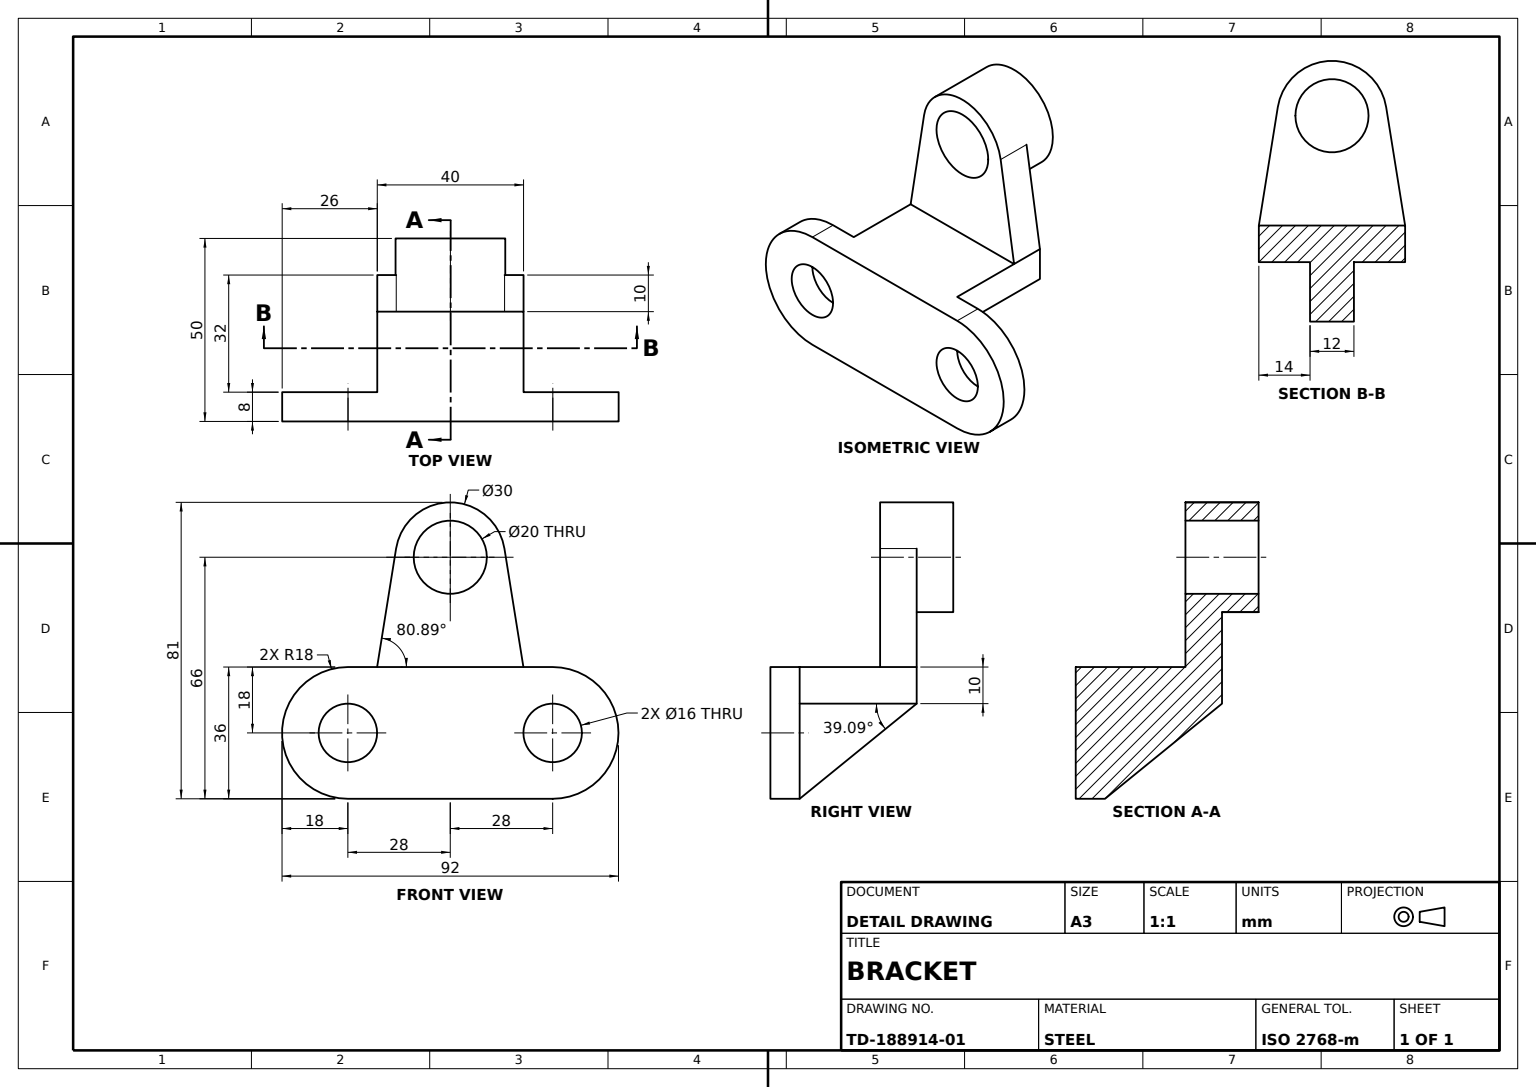
from build123d import *

# Parameters (mm, degrees)
BASE_PLATE_SKETCH_W        = 92
BASE_PLATE_SKETCH_H        = 36
BASE_PLATE_DEPTH           = 8
ROUNDED_ENDS_R18_DEPTH     = 8
UPRIGHT_LEG_DEPTH          = 10
LUG_HEAD_DEPTH             = 10
RAISED_START               = 10
ROUND_BOSS_SKETCH_R        = 15
RAISED_ROUND_BOSS_30_DEPTH = 10
BOSS_BORE_SKETCH_R         = 10
BOSS_BORE_20_DEPTH         = 20
MOUNTING_HOLES_SKETCH_R    = 8
MOUNTING_HOLES_2X_16_DEPTH = 20
RIB_DEPTH                  = 40
RIB_TRIM_CUT_1_DEPTH       = 14
RIB_TRIM_CUT_2_DEPTH       = 14


with BuildPart() as part:
    # Base Plate Sketch → Base Plate (new body)
    with BuildSketch(Plane.XY):
        with Locations((46, 18)):
            Rectangle(BASE_PLATE_SKETCH_W, BASE_PLATE_SKETCH_H)
    extrude(amount=BASE_PLATE_DEPTH)

    # Rounded Ends Sketch → Rounded Ends R18 (cut)
    with BuildSketch(Plane.XY.offset(8)):
        with BuildLine():
            Line((18, 36), (0, 36))
            Line((0, 36), (0, 18))
            ThreePointArc((0, 18), (5.272077939, 30.727922061), (18, 36))
        make_face()
        with BuildLine():
            ThreePointArc((18, 0), (5.272077939, 5.272077939), (0, 18))
            Line((0, 18), (0, 0))
            Line((0, 0), (18, 0))
        make_face()
        with BuildLine():
            Line((92, 0), (92, 18))
            ThreePointArc((92, 18), (86.727922061, 5.272077939), (74, 0))
            Line((74, 0), (92, 0))
        make_face()
        with BuildLine():
            Line((92, 36), (74, 36))
            ThreePointArc((74, 36), (86.727922061, 30.727922061), (92, 18))
            Line((92, 18), (92, 36))
        make_face()
    extrude(amount=-ROUNDED_ENDS_R18_DEPTH, mode=Mode.SUBTRACT)

    # Upright Leg Sketch → Upright Leg (add)
    with BuildSketch(Plane(origin=(0, 36, 0), x_dir=(1, 0, 0), z_dir=(0, 1, 0))):
        Polygon((46, 0), (26, 0), (26, 32), (66, 32), (66, 0), align=None)
    extrude(amount=-UPRIGHT_LEG_DEPTH)

    # Lug Head Sketch → Lug Head (add)
    with BuildSketch(Plane(origin=(0, 0, -32), x_dir=(-1, 0, 0), z_dir=(0, 0, -1))):
        with BuildLine():
            Line((-66, 36), (-26, 36))
            Line((-26, 36), (-31.189048708, 68.373967528))
            ThreePointArc((-31.189048708, 68.373967528), (-46, 81), (-60.810951292, 68.373967528))
            Line((-60.810951292, 68.373967528), (-66, 36))
        make_face()
    extrude(amount=-LUG_HEAD_DEPTH)

    # Round Boss Sketch → Raised Round Boss Ø30 (add)
    with BuildSketch(Plane(origin=(0, 0, -32), x_dir=(-1, 0, 0), z_dir=(0, 0, -1)).offset(RAISED_START)):
        with Locations((-46, 66)):
            Circle(ROUND_BOSS_SKETCH_R)
    extrude(amount=-RAISED_ROUND_BOSS_30_DEPTH)

    # Boss Bore Sketch → Boss Bore Ø20 (cut)
    with BuildSketch(Plane(origin=(0, 0, -42), x_dir=(-1, 0, 0), z_dir=(0, 0, -1))):
        with Locations((-46, 66)):
            Circle(BOSS_BORE_SKETCH_R)
    extrude(amount=-BOSS_BORE_20_DEPTH, mode=Mode.SUBTRACT)

    # Mounting Holes Sketch → Mounting Holes 2xØ16 (cut)
    with BuildSketch(Plane(origin=(0, 0, 0), x_dir=(-1, 0, 0), z_dir=(0, 0, -1))):
        with Locations((-74, 18)):
            Circle(MOUNTING_HOLES_SKETCH_R)
        with Locations((-18, 18)):
            Circle(MOUNTING_HOLES_SKETCH_R)
    extrude(amount=-MOUNTING_HOLES_2X_16_DEPTH, mode=Mode.SUBTRACT)

    # Rib Sketch → Rib (add)
    with BuildSketch(Plane.ZY.offset(-26)):
        Polygon((-32, 26), (0, 26), (0, 0), align=None)
    extrude(amount=-RIB_DEPTH)

    # Rib Trim Sketch 1 → Rib Trim Cut 1 (cut)
    with BuildSketch(Plane.ZY.offset(-26)):
        Polygon((-32, 26), (0, 26), (0, 0), align=None)
    extrude(amount=-RIB_TRIM_CUT_1_DEPTH, mode=Mode.SUBTRACT)

    # Rib Trim Sketch 2 → Rib Trim Cut 2 (cut)
    with BuildSketch(Plane(origin=(66, 0, 0), x_dir=(0, 0, -1), z_dir=(1, 0, 0))):
        Polygon((32, 26), (0, 26), (0, 0), align=None)
    extrude(amount=-RIB_TRIM_CUT_2_DEPTH, mode=Mode.SUBTRACT)


solid = part.part
